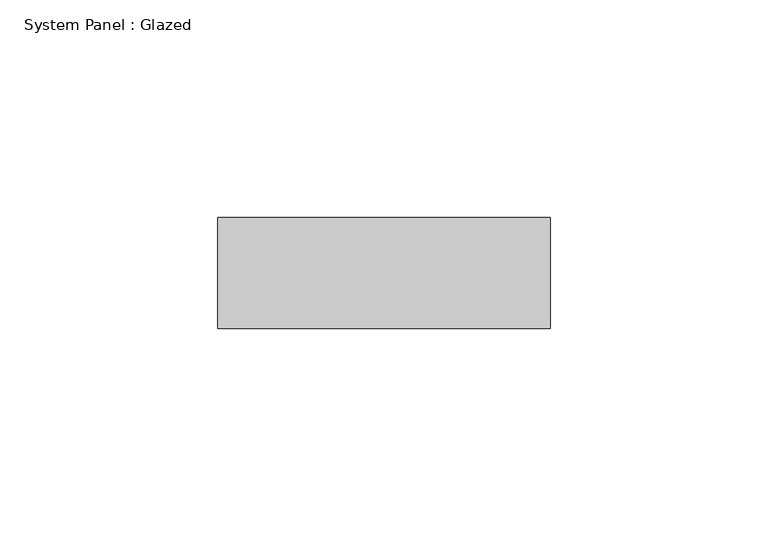
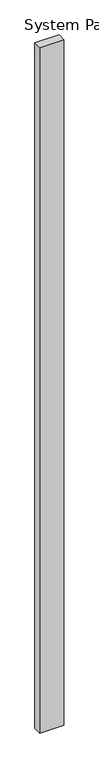
"""IFC4 building model written with IfcOpenShell, lengths in millimetres: plate geometry, System Panel : Glazed."""

from ifc_helpers import new_model, si_unit, origin, origin_with_axes, place, context, project, spatial, polyline, outline, extrude, source, transform, mapped, element, save


def system_panel_glazed_1ebf9f1f(model_context):
    return source(origin(), model_context, "Body", "SweptSolid", [
        extrude(outline(polyline([(38.1, 19.05), (-38.1, 19.05), (-38.1, 44.45), (38.1, 44.45), (38.1, 19.05)])), origin_with_axes(), (0.0, 0.0, 1.0), 2287.5875),
    ])


if __name__ == "__main__":
    model = new_model("IFC4")
    model_context = context("Model", 3, world=origin())
    ifc_project = project(units=[si_unit("LENGTHUNIT", "METRE", prefix="MILLI")], contexts=[model_context])
    site = spatial("IfcSite", under=ifc_project)
    building = spatial("IfcBuilding", under=site)
    placement = place(None, origin())
    system_panel_glazed_shape = system_panel_glazed_1ebf9f1f(model_context)
    element("IfcPlate", 1, ObjectType="System Panel : Glazed", at=placement, inside=building, context=model_context, shape_type="MappedRepresentation", body=[
        mapped(system_panel_glazed_shape, transform((0.0, 0.0, 0.0), x_axis=(1.0, 0.0, 0.0), y_axis=(0.0, 1.0, 0.0), z_axis=(0.0, 0.0, 1.0))),
    ])
    save(model, "model.ifc")

# Revit data of these elements
# Type "System Panel : Glazed"
#   Construction Type Id = "GSP4R"
#   Analytic Construction = "1/8 in Pilkington single glazing"
#   Visual Light Transmittance = 0.9
#   Solar Heat Gain Coefficient = 0.86
#   Heat Transfer Coefficient (U) = 1.18115 BTU/(h·ft²·°F)
#   Define Thermal Properties by = 1
# Element 1 (IfcPlate, "System Panel : Glazed")
#   Materials on its faces: "Glass"
# Materials
#   "Glass": class "Glass", colour RGB 0 128 192, transparency 0.75, Description = "Soda Lime Glass", Cost = 0
